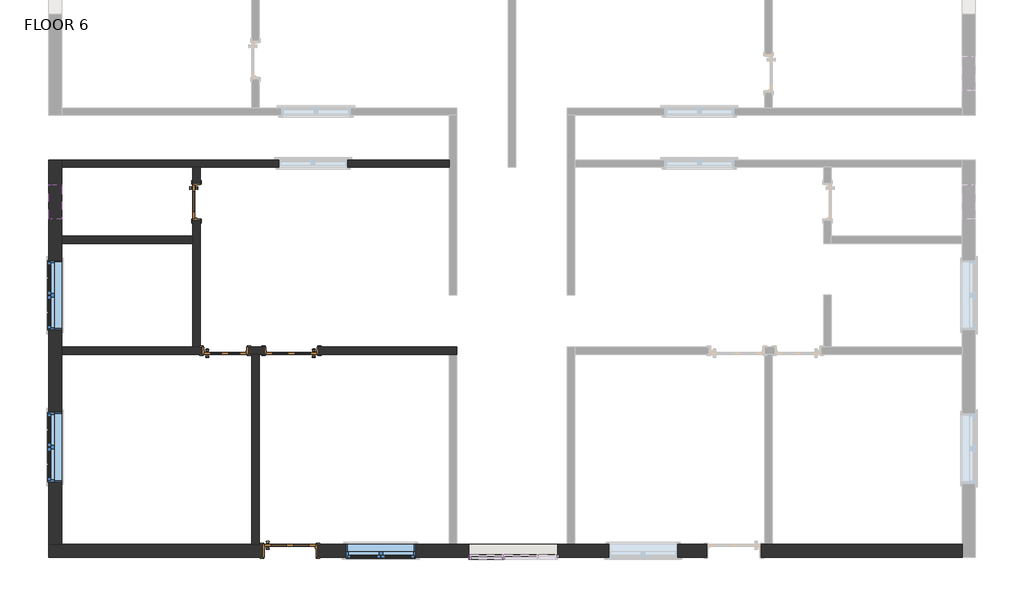
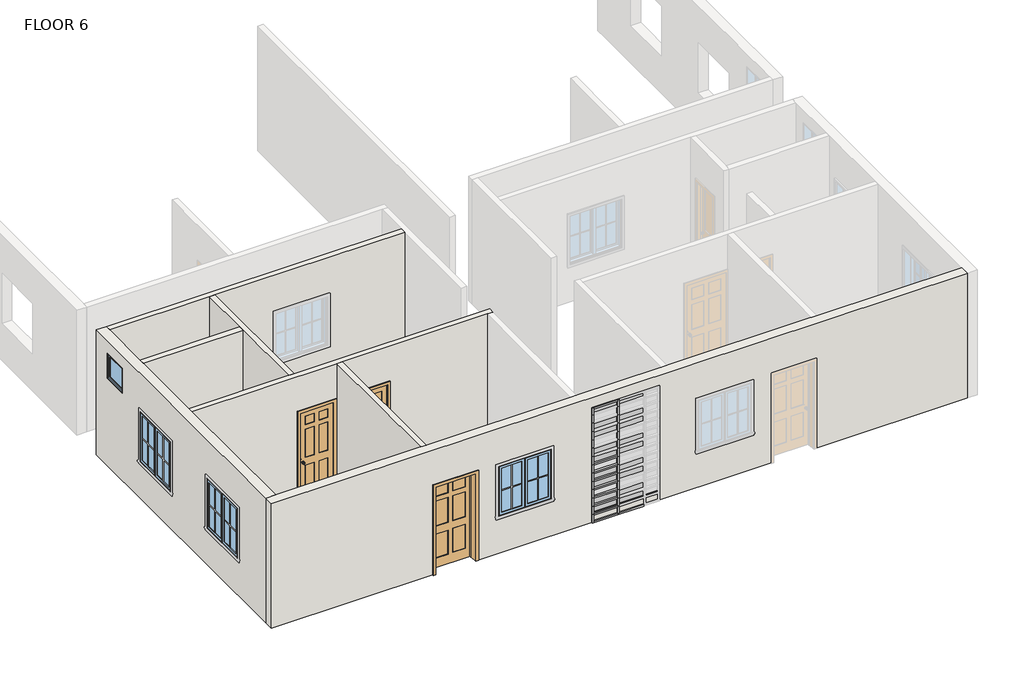
# One storey, part 1 of 4: 38 members, 20 plates, 7 walls, 4 doors, 4 windows.
"""IFC4 building model written with IfcOpenShell, lengths in millimetres."""

from ifc_helpers import new_model, si_unit, frame, origin, place, context, project, spatial, polyline, outline, extrude, faceted_brep, transform, mapped, element, save
from components import door_e337afa5, door_3b50870b, door_d86b6c54, door_03e3dfb5, member_56b223d9, member_a59c64b1, member_fa69921b, member_a67f877f, member_6a7c88b6, member_dc11c383, member_ff422208, system_panel_glazed_844a74e3, system_panel_glazed_a39216e9, system_panel_glazed_b3845325, system_panel_glazed_23b8b45c, system_panel_glazed_26c33eb0, system_panel_glazed_afc0885c, window_80340324, window_9200f5ac

model = new_model("IFC4")

# Units and contexts
model_context = context("Model", 3, world=origin())
ifc_project = project(units=[si_unit("LENGTHUNIT", "METRE", prefix="MILLI")], contexts=[model_context])

# Site, building, storey
site = spatial("IfcSite", under=ifc_project)
building = spatial("IfcBuilding", under=site)
storey = spatial("IfcBuildingStorey", under=building, Name="FLOOR 6", Elevation=9544.3725604)

# Doors
placement = place(None, origin())
door_shape = door_e337afa5(model_context)
element("IfcDoor", 1, ObjectType="Door-Interior-Single-2_Panel-Wood : 24\" x 84\"", at=placement, inside=storey, context=model_context, shape_type="MappedRepresentation", body=[
    mapped(door_shape, transform((-9830.0887331, -1548.6593836, 9544.3725604), x_axis=(0.0, -1.0, 0.0), y_axis=(1.0, 0.0, 0.0), z_axis=(0.0, 0.0, 1.0))),
])
door_2_shape = door_3b50870b(model_context)
element("IfcDoor", 2, ObjectType="Door-Interior-Single-6_Panel-Wood : 30\" x 84\"", at=placement, inside=storey, context=model_context, shape_type="MappedRepresentation", body=[
    mapped(door_2_shape, transform((-9318.9137331, -4180.7343836, 9544.3725604), x_axis=(1.0, 0.0, 0.0), y_axis=(0.0, 1.0, 0.0), z_axis=(0.0, 0.0, 1.0))),
])
door_3_shape = door_d86b6c54(model_context)
element("IfcDoor", 3, ObjectType="Door-Interior-Single-6_Panel-Wood : 36\" x 84\"", at=placement, inside=storey, context=model_context, shape_type="MappedRepresentation", body=[
    mapped(door_3_shape, transform((-8175.9137331, -7704.9843836, 9544.3725604), x_axis=(1.0, 0.0, 0.0), y_axis=(0.0, 1.0, 0.0), z_axis=(0.0, 0.0, 1.0))),
])
door_4_shape = door_03e3dfb5(model_context)
element("IfcDoor", 4, ObjectType="Door-Interior-Single-6_Panel-Wood : 36\" x 84\"", at=placement, inside=storey, context=model_context, shape_type="MappedRepresentation", body=[
    mapped(door_4_shape, transform((-8150.5137331, -4180.7343836, 9544.3725604), x_axis=(-1.0, 0.0, 0.0), y_axis=(0.0, -1.0, 0.0), z_axis=(0.0, 0.0, 1.0))),
])

# Members
member_shape = member_56b223d9(model_context)
element("IfcMember", 5, ObjectType="Rectangular Mullion : 1.5\" x 2.5\" rectangular", at=placement, inside=storey, context=model_context, shape_type="MappedRepresentation", body=[
    mapped(member_shape, transform((-4416.6334597, -7822.4593836, 9544.3725604), x_axis=(1.0, 0.0, 0.0), y_axis=(0.0, -1.0, 0.0), z_axis=(0.0, 0.0, -1.0))),
])
element("IfcMember", 6, ObjectType="Rectangular Mullion : 1.5\" x 2.5\" rectangular", at=placement, inside=storey, context=model_context, shape_type="MappedRepresentation", body=[
    mapped(member_shape, transform((-4416.6334597, -7822.4593836, 9747.5725604), x_axis=(1.0, 0.0, 0.0), y_axis=(0.0, -1.0, 0.0), z_axis=(0.0, 0.0, -1.0))),
])
element("IfcMember", 7, ObjectType="Rectangular Mullion : 1.5\" x 2.5\" rectangular", at=placement, inside=storey, context=model_context, shape_type="MappedRepresentation", body=[
    mapped(member_shape, transform((-4416.6334597, -7822.4593836, 9950.7725604), x_axis=(1.0, 0.0, 0.0), y_axis=(0.0, -1.0, 0.0), z_axis=(0.0, 0.0, -1.0))),
])
element("IfcMember", 8, ObjectType="Rectangular Mullion : 1.5\" x 2.5\" rectangular", at=placement, inside=storey, context=model_context, shape_type="MappedRepresentation", body=[
    mapped(member_shape, transform((-4416.6334597, -7822.4593836, 10153.9725604), x_axis=(1.0, 0.0, 0.0), y_axis=(0.0, -1.0, 0.0), z_axis=(0.0, 0.0, -1.0))),
])
element("IfcMember", 9, ObjectType="Rectangular Mullion : 1.5\" x 2.5\" rectangular", at=placement, inside=storey, context=model_context, shape_type="MappedRepresentation", body=[
    mapped(member_shape, transform((-4416.6334597, -7822.4593836, 10357.1725604), x_axis=(1.0, 0.0, 0.0), y_axis=(0.0, -1.0, 0.0), z_axis=(0.0, 0.0, -1.0))),
])
element("IfcMember", 10, ObjectType="Rectangular Mullion : 1.5\" x 2.5\" rectangular", at=placement, inside=storey, context=model_context, shape_type="MappedRepresentation", body=[
    mapped(member_shape, transform((-4416.6334597, -7822.4593836, 10560.3725604), x_axis=(1.0, 0.0, 0.0), y_axis=(0.0, -1.0, 0.0), z_axis=(0.0, 0.0, -1.0))),
])
element("IfcMember", 11, ObjectType="Rectangular Mullion : 1.5\" x 2.5\" rectangular", at=placement, inside=storey, context=model_context, shape_type="MappedRepresentation", body=[
    mapped(member_shape, transform((-4416.6334597, -7822.4593836, 10763.5725604), x_axis=(1.0, 0.0, 0.0), y_axis=(0.0, -1.0, 0.0), z_axis=(0.0, 0.0, -1.0))),
])
element("IfcMember", 12, ObjectType="Rectangular Mullion : 1.5\" x 2.5\" rectangular", at=placement, inside=storey, context=model_context, shape_type="MappedRepresentation", body=[
    mapped(member_shape, transform((-4416.6334597, -7822.4593836, 10966.7725604), x_axis=(1.0, 0.0, 0.0), y_axis=(0.0, -1.0, 0.0), z_axis=(0.0, 0.0, -1.0))),
])
element("IfcMember", 13, ObjectType="Rectangular Mullion : 1.5\" x 2.5\" rectangular", at=placement, inside=storey, context=model_context, shape_type="MappedRepresentation", body=[
    mapped(member_shape, transform((-4416.6334597, -7822.4593836, 11169.9725604), x_axis=(1.0, 0.0, 0.0), y_axis=(0.0, -1.0, 0.0), z_axis=(0.0, 0.0, -1.0))),
])
element("IfcMember", 14, ObjectType="Rectangular Mullion : 1.5\" x 2.5\" rectangular", at=placement, inside=storey, context=model_context, shape_type="MappedRepresentation", body=[
    mapped(member_shape, transform((-4416.6334597, -7822.4593836, 11373.1725604), x_axis=(1.0, 0.0, 0.0), y_axis=(0.0, -1.0, 0.0), z_axis=(0.0, 0.0, -1.0))),
])
element("IfcMember", 15, ObjectType="Rectangular Mullion : 1.5\" x 2.5\" rectangular", at=placement, inside=storey, context=model_context, shape_type="MappedRepresentation", body=[
    mapped(member_shape, transform((-4416.6334597, -7822.4593836, 11576.3725604), x_axis=(1.0, 0.0, 0.0), y_axis=(0.0, -1.0, 0.0), z_axis=(0.0, 0.0, -1.0))),
])
element("IfcMember", 16, ObjectType="Rectangular Mullion : 1.5\" x 2.5\" rectangular", at=placement, inside=storey, context=model_context, shape_type="MappedRepresentation", body=[
    mapped(member_shape, transform((-4416.6334597, -7822.4593836, 11779.5725604), x_axis=(1.0, 0.0, 0.0), y_axis=(0.0, -1.0, 0.0), z_axis=(0.0, 0.0, -1.0))),
])
element("IfcMember", 17, ObjectType="Rectangular Mullion : 1.5\" x 2.5\" rectangular", at=placement, inside=storey, context=model_context, shape_type="MappedRepresentation", body=[
    mapped(member_shape, transform((-4416.6334597, -7822.4593836, 11982.7725604), x_axis=(1.0, 0.0, 0.0), y_axis=(0.0, -1.0, 0.0), z_axis=(0.0, 0.0, -1.0))),
])
member_2_shape = member_a59c64b1(model_context)
element("IfcMember", 18, ObjectType="Rectangular Mullion : 1.5\" x 2.5\" rectangular", at=placement, inside=storey, context=model_context, shape_type="MappedRepresentation", body=[
    mapped(member_2_shape, transform((-4416.6334597, -7822.4593836, 12185.9725604), x_axis=(1.0, 0.0, 0.0), y_axis=(0.0, -1.0, 0.0), z_axis=(0.0, 0.0, -1.0))),
])
member_3_shape = member_fa69921b(model_context)
element("IfcMember", 19, ObjectType="Rectangular Mullion : 1.5\" x 2.5\" rectangular", at=placement, inside=storey, context=model_context, shape_type="MappedRepresentation", body=[
    mapped(member_3_shape, transform((-4435.6834597, -7822.4593836, 12351.7551755), x_axis=(0.0, 0.0, 1.0), y_axis=(0.0, -1.0, 0.0), z_axis=(1.0, 0.0, 0.0))),
])
element("IfcMember", 20, ObjectType="Rectangular Mullion : 1.5\" x 2.5\" rectangular", at=placement, inside=storey, context=model_context, shape_type="MappedRepresentation", body=[
    mapped(member_3_shape, transform((-4988.13346, -7822.4593836, 9544.3725604), x_axis=(0.0, 0.0, -1.0), y_axis=(0.0, -1.0, 0.0), z_axis=(-1.0, 0.0, 0.0))),
])
member_4_shape = member_a67f877f(model_context)
element("IfcMember", 21, ObjectType="Rectangular Mullion : 1.5\" x 2.5\" rectangular", at=placement, inside=storey, context=model_context, shape_type="MappedRepresentation", body=[
    mapped(member_4_shape, transform((-4397.5834597, -7822.4593836, 9544.3725604), x_axis=(0.0, 0.0, -1.0), y_axis=(0.0, -1.0, 0.0), z_axis=(-1.0, 0.0, 0.0))),
])
member_5_shape = member_6a7c88b6(model_context)
element("IfcMember", 22, ObjectType="Rectangular Mullion : 1.5\" x 2.5\" rectangular", at=placement, inside=storey, context=model_context, shape_type="MappedRepresentation", body=[
    mapped(member_5_shape, transform((-4435.6834597, -7822.4593836, 9747.5725604), x_axis=(0.0, 0.0, 1.0), y_axis=(0.0, -1.0, 0.0), z_axis=(1.0, 0.0, 0.0))),
])
element("IfcMember", 23, ObjectType="Rectangular Mullion : 1.5\" x 2.5\" rectangular", at=placement, inside=storey, context=model_context, shape_type="MappedRepresentation", body=[
    mapped(member_5_shape, transform((-4435.6834597, -7822.4593836, 9950.7725604), x_axis=(0.0, 0.0, 1.0), y_axis=(0.0, -1.0, 0.0), z_axis=(1.0, 0.0, 0.0))),
])
element("IfcMember", 24, ObjectType="Rectangular Mullion : 1.5\" x 2.5\" rectangular", at=placement, inside=storey, context=model_context, shape_type="MappedRepresentation", body=[
    mapped(member_5_shape, transform((-4435.6834597, -7822.4593836, 10153.9725604), x_axis=(0.0, 0.0, 1.0), y_axis=(0.0, -1.0, 0.0), z_axis=(1.0, 0.0, 0.0))),
])
element("IfcMember", 25, ObjectType="Rectangular Mullion : 1.5\" x 2.5\" rectangular", at=placement, inside=storey, context=model_context, shape_type="MappedRepresentation", body=[
    mapped(member_5_shape, transform((-4435.6834597, -7822.4593836, 10357.1725604), x_axis=(0.0, 0.0, 1.0), y_axis=(0.0, -1.0, 0.0), z_axis=(1.0, 0.0, 0.0))),
])
element("IfcMember", 26, ObjectType="Rectangular Mullion : 1.5\" x 2.5\" rectangular", at=placement, inside=storey, context=model_context, shape_type="MappedRepresentation", body=[
    mapped(member_5_shape, transform((-4435.6834597, -7822.4593836, 10560.3725604), x_axis=(0.0, 0.0, 1.0), y_axis=(0.0, -1.0, 0.0), z_axis=(1.0, 0.0, 0.0))),
])
element("IfcMember", 27, ObjectType="Rectangular Mullion : 1.5\" x 2.5\" rectangular", at=placement, inside=storey, context=model_context, shape_type="MappedRepresentation", body=[
    mapped(member_5_shape, transform((-4435.6834597, -7822.4593836, 10763.5725604), x_axis=(0.0, 0.0, 1.0), y_axis=(0.0, -1.0, 0.0), z_axis=(1.0, 0.0, 0.0))),
])
element("IfcMember", 28, ObjectType="Rectangular Mullion : 1.5\" x 2.5\" rectangular", at=placement, inside=storey, context=model_context, shape_type="MappedRepresentation", body=[
    mapped(member_5_shape, transform((-4435.6834597, -7822.4593836, 10966.7725604), x_axis=(0.0, 0.0, 1.0), y_axis=(0.0, -1.0, 0.0), z_axis=(1.0, 0.0, 0.0))),
])
member_6_shape = member_dc11c383(model_context)
element("IfcMember", 29, ObjectType="Rectangular Mullion : 1.5\" x 2.5\" rectangular", at=placement, inside=storey, context=model_context, shape_type="MappedRepresentation", body=[
    mapped(member_6_shape, transform((-5026.23346, -7822.4593836, 12351.7551755), x_axis=(-1.0, 0.0, 0.0), y_axis=(0.0, -1.0, 0.0), z_axis=(0.0, 0.0, 1.0))),
])
member_7_shape = member_ff422208(model_context)
element("IfcMember", 30, ObjectType="Rectangular Mullion : 1.5\" x 2.5\" rectangular", at=placement, inside=storey, context=model_context, shape_type="MappedRepresentation", body=[
    mapped(member_7_shape, transform((-5026.23346, -7822.4593836, 9747.5725604), x_axis=(-1.0, 0.0, 0.0), y_axis=(0.0, -1.0, 0.0), z_axis=(0.0, 0.0, 1.0))),
])
element("IfcMember", 31, ObjectType="Rectangular Mullion : 1.5\" x 2.5\" rectangular", at=placement, inside=storey, context=model_context, shape_type="MappedRepresentation", body=[
    mapped(member_7_shape, transform((-5026.23346, -7822.4593836, 9950.7725604), x_axis=(-1.0, 0.0, 0.0), y_axis=(0.0, -1.0, 0.0), z_axis=(0.0, 0.0, 1.0))),
])
element("IfcMember", 32, ObjectType="Rectangular Mullion : 1.5\" x 2.5\" rectangular", at=placement, inside=storey, context=model_context, shape_type="MappedRepresentation", body=[
    mapped(member_7_shape, transform((-5026.23346, -7822.4593836, 10153.9725604), x_axis=(-1.0, 0.0, 0.0), y_axis=(0.0, -1.0, 0.0), z_axis=(0.0, 0.0, 1.0))),
])
element("IfcMember", 33, ObjectType="Rectangular Mullion : 1.5\" x 2.5\" rectangular", at=placement, inside=storey, context=model_context, shape_type="MappedRepresentation", body=[
    mapped(member_7_shape, transform((-5026.23346, -7822.4593836, 10357.1725604), x_axis=(-1.0, 0.0, 0.0), y_axis=(0.0, -1.0, 0.0), z_axis=(0.0, 0.0, 1.0))),
])
element("IfcMember", 34, ObjectType="Rectangular Mullion : 1.5\" x 2.5\" rectangular", at=placement, inside=storey, context=model_context, shape_type="MappedRepresentation", body=[
    mapped(member_7_shape, transform((-5026.23346, -7822.4593836, 10560.3725604), x_axis=(-1.0, 0.0, 0.0), y_axis=(0.0, -1.0, 0.0), z_axis=(0.0, 0.0, 1.0))),
])
element("IfcMember", 35, ObjectType="Rectangular Mullion : 1.5\" x 2.5\" rectangular", at=placement, inside=storey, context=model_context, shape_type="MappedRepresentation", body=[
    mapped(member_7_shape, transform((-5026.23346, -7822.4593836, 10763.5725604), x_axis=(-1.0, 0.0, 0.0), y_axis=(0.0, -1.0, 0.0), z_axis=(0.0, 0.0, 1.0))),
])
element("IfcMember", 36, ObjectType="Rectangular Mullion : 1.5\" x 2.5\" rectangular", at=placement, inside=storey, context=model_context, shape_type="MappedRepresentation", body=[
    mapped(member_7_shape, transform((-5026.23346, -7822.4593836, 10966.7725604), x_axis=(-1.0, 0.0, 0.0), y_axis=(0.0, -1.0, 0.0), z_axis=(0.0, 0.0, 1.0))),
])
element("IfcMember", 37, ObjectType="Rectangular Mullion : 1.5\" x 2.5\" rectangular", at=placement, inside=storey, context=model_context, shape_type="MappedRepresentation", body=[
    mapped(member_7_shape, transform((-5026.23346, -7822.4593836, 11169.9725604), x_axis=(-1.0, 0.0, 0.0), y_axis=(0.0, -1.0, 0.0), z_axis=(0.0, 0.0, 1.0))),
])
element("IfcMember", 38, ObjectType="Rectangular Mullion : 1.5\" x 2.5\" rectangular", at=placement, inside=storey, context=model_context, shape_type="MappedRepresentation", body=[
    mapped(member_7_shape, transform((-5026.23346, -7822.4593836, 11373.1725604), x_axis=(-1.0, 0.0, 0.0), y_axis=(0.0, -1.0, 0.0), z_axis=(0.0, 0.0, 1.0))),
])
element("IfcMember", 39, ObjectType="Rectangular Mullion : 1.5\" x 2.5\" rectangular", at=placement, inside=storey, context=model_context, shape_type="MappedRepresentation", body=[
    mapped(member_7_shape, transform((-5026.23346, -7822.4593836, 11576.3725604), x_axis=(-1.0, 0.0, 0.0), y_axis=(0.0, -1.0, 0.0), z_axis=(0.0, 0.0, 1.0))),
])
element("IfcMember", 40, ObjectType="Rectangular Mullion : 1.5\" x 2.5\" rectangular", at=placement, inside=storey, context=model_context, shape_type="MappedRepresentation", body=[
    mapped(member_7_shape, transform((-5026.23346, -7822.4593836, 11779.5725604), x_axis=(-1.0, 0.0, 0.0), y_axis=(0.0, -1.0, 0.0), z_axis=(0.0, 0.0, 1.0))),
])
element("IfcMember", 41, ObjectType="Rectangular Mullion : 1.5\" x 2.5\" rectangular", at=placement, inside=storey, context=model_context, shape_type="MappedRepresentation", body=[
    mapped(member_7_shape, transform((-5026.23346, -7822.4593836, 11982.7725604), x_axis=(-1.0, 0.0, 0.0), y_axis=(0.0, -1.0, 0.0), z_axis=(0.0, 0.0, 1.0))),
])
element("IfcMember", 42, ObjectType="Rectangular Mullion : 1.5\" x 2.5\" rectangular", at=placement, inside=storey, context=model_context, shape_type="MappedRepresentation", body=[
    mapped(member_7_shape, transform((-5026.23346, -7822.4593836, 12185.9725604), x_axis=(-1.0, 0.0, 0.0), y_axis=(0.0, -1.0, 0.0), z_axis=(0.0, 0.0, 1.0))),
])

# Plates
system_panel_glazed_shape = system_panel_glazed_844a74e3(model_context)
element("IfcPlate", 43, ObjectType="System Panel : Glazed", at=placement, inside=storey, context=model_context, shape_type="MappedRepresentation", body=[
    mapped(system_panel_glazed_shape, transform((-4711.9084599, -7822.4593836, 9582.4725604), x_axis=(1.0, 0.0, 0.0), y_axis=(0.0, 1.0, 0.0), z_axis=(0.0, 0.0, 1.0))),
])
system_panel_glazed_2_shape = system_panel_glazed_a39216e9(model_context)
element("IfcPlate", 44, ObjectType="System Panel : Glazed", at=placement, inside=storey, context=model_context, shape_type="MappedRepresentation", body=[
    mapped(system_panel_glazed_2_shape, transform((-4111.8334597, -7822.4593836, 9582.4725604), x_axis=(1.0, 0.0, 0.0), y_axis=(0.0, 1.0, 0.0), z_axis=(0.0, 0.0, 1.0))),
])
system_panel_glazed_3_shape = system_panel_glazed_b3845325(model_context)
element("IfcPlate", 45, ObjectType="System Panel : Glazed", at=placement, inside=storey, context=model_context, shape_type="MappedRepresentation", body=[
    mapped(system_panel_glazed_3_shape, transform((-4711.9084599, -7822.4593836, 9766.6225604), x_axis=(1.0, 0.0, 0.0), y_axis=(0.0, 1.0, 0.0), z_axis=(0.0, 0.0, 1.0))),
])
element("IfcPlate", 46, ObjectType="System Panel : Glazed", at=placement, inside=storey, context=model_context, shape_type="MappedRepresentation", body=[
    mapped(system_panel_glazed_3_shape, transform((-4711.9084599, -7822.4593836, 9969.8225604), x_axis=(1.0, 0.0, 0.0), y_axis=(0.0, 1.0, 0.0), z_axis=(0.0, 0.0, 1.0))),
])
element("IfcPlate", 47, ObjectType="System Panel : Glazed", at=placement, inside=storey, context=model_context, shape_type="MappedRepresentation", body=[
    mapped(system_panel_glazed_3_shape, transform((-4711.9084599, -7822.4593836, 10376.2225604), x_axis=(1.0, 0.0, 0.0), y_axis=(0.0, 1.0, 0.0), z_axis=(0.0, 0.0, 1.0))),
])
element("IfcPlate", 48, ObjectType="System Panel : Glazed", at=placement, inside=storey, context=model_context, shape_type="MappedRepresentation", body=[
    mapped(system_panel_glazed_3_shape, transform((-4711.9084599, -7822.4593836, 10579.4225604), x_axis=(1.0, 0.0, 0.0), y_axis=(0.0, 1.0, 0.0), z_axis=(0.0, 0.0, 1.0))),
])
element("IfcPlate", 49, ObjectType="System Panel : Glazed", at=placement, inside=storey, context=model_context, shape_type="MappedRepresentation", body=[
    mapped(system_panel_glazed_3_shape, transform((-4711.9084599, -7822.4593836, 10985.8225604), x_axis=(1.0, 0.0, 0.0), y_axis=(0.0, 1.0, 0.0), z_axis=(0.0, 0.0, 1.0))),
])
element("IfcPlate", 50, ObjectType="System Panel : Glazed", at=placement, inside=storey, context=model_context, shape_type="MappedRepresentation", body=[
    mapped(system_panel_glazed_3_shape, transform((-4711.9084599, -7822.4593836, 11189.0225604), x_axis=(1.0, 0.0, 0.0), y_axis=(0.0, 1.0, 0.0), z_axis=(0.0, 0.0, 1.0))),
])
element("IfcPlate", 51, ObjectType="System Panel : Glazed", at=placement, inside=storey, context=model_context, shape_type="MappedRepresentation", body=[
    mapped(system_panel_glazed_3_shape, transform((-4711.9084599, -7822.4593836, 11595.4225604), x_axis=(1.0, 0.0, 0.0), y_axis=(0.0, 1.0, 0.0), z_axis=(0.0, 0.0, 1.0))),
])
element("IfcPlate", 52, ObjectType="System Panel : Glazed", at=placement, inside=storey, context=model_context, shape_type="MappedRepresentation", body=[
    mapped(system_panel_glazed_3_shape, transform((-4711.9084599, -7822.4593836, 11798.6225604), x_axis=(1.0, 0.0, 0.0), y_axis=(0.0, 1.0, 0.0), z_axis=(0.0, 0.0, 1.0))),
])
system_panel_glazed_4_shape = system_panel_glazed_23b8b45c(model_context)
element("IfcPlate", 53, ObjectType="System Panel : Glazed", at=placement, inside=storey, context=model_context, shape_type="MappedRepresentation", body=[
    mapped(system_panel_glazed_4_shape, transform((-4111.8334597, -7822.4593836, 9766.6225604), x_axis=(1.0, 0.0, 0.0), y_axis=(0.0, 1.0, 0.0), z_axis=(0.0, 0.0, 1.0))),
])
element("IfcPlate", 54, ObjectType="System Panel : Glazed", at=placement, inside=storey, context=model_context, shape_type="MappedRepresentation", body=[
    mapped(system_panel_glazed_4_shape, transform((-4111.8334597, -7822.4593836, 9969.8225604), x_axis=(1.0, 0.0, 0.0), y_axis=(0.0, 1.0, 0.0), z_axis=(0.0, 0.0, 1.0))),
])
element("IfcPlate", 55, ObjectType="System Panel : Glazed", at=placement, inside=storey, context=model_context, shape_type="MappedRepresentation", body=[
    mapped(system_panel_glazed_4_shape, transform((-4111.8334597, -7822.4593836, 10376.2225604), x_axis=(1.0, 0.0, 0.0), y_axis=(0.0, 1.0, 0.0), z_axis=(0.0, 0.0, 1.0))),
])
element("IfcPlate", 56, ObjectType="System Panel : Glazed", at=placement, inside=storey, context=model_context, shape_type="MappedRepresentation", body=[
    mapped(system_panel_glazed_4_shape, transform((-4111.8334597, -7822.4593836, 10579.4225604), x_axis=(1.0, 0.0, 0.0), y_axis=(0.0, 1.0, 0.0), z_axis=(0.0, 0.0, 1.0))),
])
element("IfcPlate", 57, ObjectType="System Panel : Glazed", at=placement, inside=storey, context=model_context, shape_type="MappedRepresentation", body=[
    mapped(system_panel_glazed_4_shape, transform((-4111.8334597, -7822.4593836, 10985.8225604), x_axis=(1.0, 0.0, 0.0), y_axis=(0.0, 1.0, 0.0), z_axis=(0.0, 0.0, 1.0))),
])
element("IfcPlate", 58, ObjectType="System Panel : Glazed", at=placement, inside=storey, context=model_context, shape_type="MappedRepresentation", body=[
    mapped(system_panel_glazed_4_shape, transform((-4111.8334597, -7822.4593836, 11189.0225604), x_axis=(1.0, 0.0, 0.0), y_axis=(0.0, 1.0, 0.0), z_axis=(0.0, 0.0, 1.0))),
])
element("IfcPlate", 59, ObjectType="System Panel : Glazed", at=placement, inside=storey, context=model_context, shape_type="MappedRepresentation", body=[
    mapped(system_panel_glazed_4_shape, transform((-4111.8334597, -7822.4593836, 11595.4225604), x_axis=(1.0, 0.0, 0.0), y_axis=(0.0, 1.0, 0.0), z_axis=(0.0, 0.0, 1.0))),
])
element("IfcPlate", 60, ObjectType="System Panel : Glazed", at=placement, inside=storey, context=model_context, shape_type="MappedRepresentation", body=[
    mapped(system_panel_glazed_4_shape, transform((-4111.8334597, -7822.4593836, 11798.6225604), x_axis=(1.0, 0.0, 0.0), y_axis=(0.0, 1.0, 0.0), z_axis=(0.0, 0.0, 1.0))),
])
system_panel_glazed_5_shape = system_panel_glazed_26c33eb0(model_context)
element("IfcPlate", 61, ObjectType="System Panel : Glazed", at=placement, inside=storey, context=model_context, shape_type="MappedRepresentation", body=[
    mapped(system_panel_glazed_5_shape, transform((-4711.9084599, -7822.4593836, 12205.0225604), x_axis=(1.0, 0.0, 0.0), y_axis=(0.0, 1.0, 0.0), z_axis=(0.0, 0.0, 1.0))),
])
system_panel_glazed_6_shape = system_panel_glazed_afc0885c(model_context)
element("IfcPlate", 62, ObjectType="System Panel : Glazed", at=placement, inside=storey, context=model_context, shape_type="MappedRepresentation", body=[
    mapped(system_panel_glazed_6_shape, transform((-4111.8334597, -7822.4593836, 12205.0225604), x_axis=(1.0, 0.0, 0.0), y_axis=(0.0, 1.0, 0.0), z_axis=(0.0, 0.0, 1.0))),
])

# Walls
element("IfcWall", 63, ObjectType="Inner Wall 5\"", at=placement, inside=storey, context=model_context, shape_type="Brep", body=[
    faceted_brep([(-12201.8137331, -939.0593836, 9544.3725604), (-9890.4137331, -939.0593836, 9544.3725604), (-9763.4137331, -939.0593836, 9544.3725604), (-5369.2137331, -939.0593836, 9544.3725604), (-5369.2137331, -939.0593836, 12592.3725604), (-9763.4137331, -939.0593836, 12592.3725604), (-9890.4137331, -939.0593836, 12592.3725604), (-12201.8137331, -939.0593836, 12592.3725604), (-7159.9137331, -939.0593836, 11677.9725604), (-7159.9137331, -939.0593836, 10458.7725604), (-8379.1137331, -939.0593836, 10458.7725604), (-8379.1137331, -939.0593836, 11677.9725604), (-12201.8137331, -812.0593836, 9544.3725604), (-12201.8137331, -812.0593836, 12592.3725604), (-5369.2137331, -812.0593836, 12592.3725604), (-5369.2137331, -812.0593836, 9544.3725604), (-7159.9137331, -812.0593836, 11677.9725604), (-8379.1137331, -812.0593836, 11677.9725604), (-8379.1137331, -812.0593836, 10458.7725604), (-7159.9137331, -812.0593836, 10458.7725604)], [[[0, 1, 2, 3, 4, 5, 6, 7], [8, 9, 10, 11]], [[12, 13, 14, 15], [16, 17, 18, 19]], [[3, 2, 1, 0, 12, 15]], [[7, 6, 5, 4, 14, 13]], [[0, 7, 13, 12]], [[4, 3, 15, 14]], [[9, 8, 16, 19]], [[10, 9, 19, 18]], [[11, 10, 18, 17]], [[8, 11, 17, 16]]]),
])
element("IfcWall", 64, ObjectType="Inner Wall 5\"", at=placement, inside=storey, context=model_context, shape_type="SweptSolid", body=[
    extrude(outline(polyline([(-8722.0137331, -4241.0593836), (-8722.0137331, -7593.8593836), (-8849.0137331, -7593.8593836), (-8849.0137331, -4241.0593836), (-8722.0137331, -4241.0593836)])), frame((0.0, 0.0, 9544.3725604), z_axis=(0.0, 0.0, 1.0), x_axis=(1.0, 0.0, 0.0)), (0.0, 0.0, 1.0), 3048.0),
])
element("IfcWall", 65, ObjectType="Inner Wall 5\"", at=placement, inside=storey, context=model_context, shape_type="Brep", body=[
    faceted_brep([(-12201.8137331, -4114.0593836, 12592.3725604), (-9890.4137331, -4114.0593836, 12592.3725604), (-9763.4137331, -4114.0593836, 12592.3725604), (-5242.2137331, -4114.0593836, 12592.3725604), (-5242.2137331, -4114.0593836, 9544.3725604), (-7667.9137331, -4114.0593836, 9544.3725604), (-7667.9137331, -4114.0593836, 11703.3725604), (-8633.1137331, -4114.0593836, 11703.3725604), (-8633.1137331, -4114.0593836, 9544.3725604), (-8912.5137331, -4114.0593836, 9544.3725604), (-8912.5137331, -4114.0593836, 11703.3725604), (-9725.3137331, -4114.0593836, 11703.3725604), (-9725.3137331, -4114.0593836, 9544.3725604), (-9763.4137331, -4114.0593836, 9544.3725604), (-9890.4137331, -4114.0593836, 9544.3725604), (-12201.8137331, -4114.0593836, 9544.3725604), (-5242.2137331, -4241.0593836, 12592.3725604), (-5369.2137331, -4241.0593836, 12592.3725604), (-8722.0137331, -4241.0593836, 12592.3725604), (-8849.0137331, -4241.0593836, 12592.3725604), (-12201.8137331, -4241.0593836, 12592.3725604), (-12201.8137331, -4241.0593836, 9544.3725604), (-9725.3137331, -4241.0593836, 9544.3725604), (-9725.3137331, -4241.0593836, 11703.3725604), (-8912.5137331, -4241.0593836, 11703.3725604), (-8912.5137331, -4241.0593836, 9544.3725604), (-8849.0137331, -4241.0593836, 9544.3725604), (-8722.0137331, -4241.0593836, 9544.3725604), (-8633.1137331, -4241.0593836, 9544.3725604), (-8633.1137331, -4241.0593836, 11703.3725604), (-7667.9137331, -4241.0593836, 11703.3725604), (-7667.9137331, -4241.0593836, 9544.3725604), (-5369.2137331, -4241.0593836, 9544.3725604), (-5242.2137331, -4241.0593836, 9544.3725604)], [[[0, 1, 2, 3, 4, 5, 6, 7, 8, 9, 10, 11, 12, 13, 14, 15]], [[16, 17, 18, 19, 20, 21, 22, 23, 24, 25, 26, 27, 28, 29, 30, 31, 32, 33]], [[21, 15, 14, 13, 12, 22]], [[4, 33, 32, 31, 5]], [[25, 9, 8, 28, 27, 26]], [[3, 2, 1, 0, 20, 19, 18, 17, 16]], [[0, 15, 21, 20]], [[4, 3, 16, 33]], [[10, 9, 25, 24]], [[11, 10, 24, 23]], [[12, 11, 23, 22]], [[7, 29, 28, 8]], [[29, 7, 6, 30]], [[30, 6, 5, 31]]]),
])
element("IfcWall", 66, ObjectType="Inner Wall 5\"", at=placement, inside=storey, context=model_context, shape_type="Brep", body=[
    faceted_brep([(-9763.4137331, -939.0593836, 12592.3725604), (-9763.4137331, -4114.0593836, 12592.3725604), (-9763.4137331, -4114.0593836, 9544.3725604), (-9763.4137331, -1878.8593836, 9544.3725604), (-9763.4137331, -1878.8593836, 11703.3725604), (-9763.4137331, -1218.4593836, 11703.3725604), (-9763.4137331, -1218.4593836, 9544.3725604), (-9763.4137331, -939.0593836, 9544.3725604), (-9890.4137331, -4114.0593836, 12592.3725604), (-9890.4137331, -2285.2593836, 12592.3725604), (-9890.4137331, -2158.2593836, 12592.3725604), (-9890.4137331, -939.0593836, 12592.3725604), (-9890.4137331, -939.0593836, 9544.3725604), (-9890.4137331, -1218.4593836, 9544.3725604), (-9890.4137331, -1218.4593836, 11703.3725604), (-9890.4137331, -1878.8593836, 11703.3725604), (-9890.4137331, -1878.8593836, 9544.3725604), (-9890.4137331, -2158.2593836, 9544.3725604), (-9890.4137331, -2285.2593836, 9544.3725604), (-9890.4137331, -4114.0593836, 9544.3725604)], [[[0, 1, 2, 3, 4, 5, 6, 7]], [[8, 9, 10, 11, 12, 13, 14, 15, 16, 17, 18, 19]], [[2, 19, 18, 17, 16, 3]], [[12, 7, 6, 13]], [[1, 0, 11, 10, 9, 8]], [[2, 1, 8, 19]], [[0, 7, 12, 11]], [[15, 4, 3, 16]], [[4, 15, 14, 5]], [[5, 14, 13, 6]]]),
])
element("IfcWall", 67, ObjectType="Inner Wall 5\"", at=placement, inside=storey, context=model_context, shape_type="SweptSolid", body=[
    extrude(outline(polyline([(-12201.8137331, -2158.2593836), (-9890.4137331, -2158.2593836), (-9890.4137331, -2285.2593836), (-12201.8137331, -2285.2593836), (-12201.8137331, -2158.2593836)])), frame((0.0, 0.0, 9544.3725604), z_axis=(0.0, 0.0, 1.0), x_axis=(1.0, 0.0, 0.0)), (0.0, 0.0, 1.0), 3048.0),
])
element("IfcWall", 68, ObjectType="outer wall 9\"", at=placement, inside=storey, context=model_context, shape_type="Brep", body=[
    faceted_brep([(3673.1862669, -7822.4593836, 12592.3725604), (-12430.4137331, -7822.4593836, 12592.3725604), (-12430.4137331, -7822.4593836, 9544.3725604), (-8658.5137331, -7822.4593836, 9544.3725604), (-8658.5137331, -7822.4593836, 11703.3725604), (-7693.3137331, -7822.4593836, 11703.3725604), (-7693.3137331, -7822.4593836, 9544.3725604), (-835.3137331, -7822.4593836, 9544.3725604), (-835.3137331, -7822.4593836, 11703.3725604), (129.8862669, -7822.4593836, 11703.3725604), (129.8862669, -7822.4593836, 9544.3725604), (3673.1862669, -7822.4593836, 9544.3725604), (-2562.5137331, -7822.4593836, 11677.9725604), (-1343.3137331, -7822.4593836, 11677.9725604), (-1343.3137331, -7822.4593836, 10458.7725604), (-2562.5137331, -7822.4593836, 10458.7725604), (-7185.3137331, -7822.4593836, 11677.9725604), (-5966.1137331, -7822.4593836, 11677.9725604), (-5966.1137331, -7822.4593836, 10458.7725604), (-7185.3137331, -7822.4593836, 10458.7725604), (-5026.23346, -7822.4593836, 12351.7551755), (-3461.6513929, -7822.4593836, 12351.7551755), (-3461.6513929, -7822.4593836, 9778.8868874), (-5026.23346, -7822.4593836, 9778.8868874), (-12430.4137331, -7593.8593836, 12592.3725604), (-12201.8137331, -7593.8593836, 12592.3725604), (-8849.0137331, -7593.8593836, 12592.3725604), (-8722.0137331, -7593.8593836, 12592.3725604), (-5369.2137331, -7593.8593836, 12592.3725604), (-5242.2137331, -7593.8593836, 12592.3725604), (-3286.4137331, -7593.8593836, 12592.3725604), (-3159.4137331, -7593.8593836, 12592.3725604), (193.3862669, -7593.8593836, 12592.3725604), (320.3862669, -7593.8593836, 12592.3725604), (3673.1862669, -7593.8593836, 12592.3725604), (3673.1862669, -7593.8593836, 9544.3725604), (320.3862669, -7593.8593836, 9544.3725604), (193.3862669, -7593.8593836, 9544.3725604), (129.8862669, -7593.8593836, 9544.3725604), (129.8862669, -7593.8593836, 11703.3725604), (-835.3137331, -7593.8593836, 11703.3725604), (-835.3137331, -7593.8593836, 9544.3725604), (-3159.4137331, -7593.8593836, 9544.3725604), (-3286.4137331, -7593.8593836, 9544.3725604), (-5242.2137331, -7593.8593836, 9544.3725604), (-5369.2137331, -7593.8593836, 9544.3725604), (-7693.3137331, -7593.8593836, 9544.3725604), (-7693.3137331, -7593.8593836, 11703.3725604), (-8658.5137331, -7593.8593836, 11703.3725604), (-8658.5137331, -7593.8593836, 9544.3725604), (-8722.0137331, -7593.8593836, 9544.3725604), (-8849.0137331, -7593.8593836, 9544.3725604), (-12201.8137331, -7593.8593836, 9544.3725604), (-12430.4137331, -7593.8593836, 9544.3725604), (-2562.5137331, -7593.8593836, 11677.9725604), (-2562.5137331, -7593.8593836, 10458.7725604), (-1343.3137331, -7593.8593836, 10458.7725604), (-1343.3137331, -7593.8593836, 11677.9725604), (-7185.3137331, -7593.8593836, 11677.9725604), (-7185.3137331, -7593.8593836, 10458.7725604), (-5966.1137331, -7593.8593836, 10458.7725604), (-5966.1137331, -7593.8593836, 11677.9725604), (-3461.6513929, -7593.8593836, 12351.7551755), (-5026.23346, -7593.8593836, 12351.7551755), (-5026.23346, -7593.8593836, 9778.8868874), (-3461.6513929, -7593.8593836, 9778.8868874)], [[[0, 1, 2, 3, 4, 5, 6, 7, 8, 9, 10, 11], [12, 13, 14, 15], [16, 17, 18, 19], [20, 21, 22, 23]], [[24, 25, 26, 27, 28, 29, 30, 31, 32, 33, 34, 35, 36, 37, 38, 39, 40, 41, 42, 43, 44, 45, 46, 47, 48, 49, 50, 51, 52, 53], [54, 55, 56, 57], [58, 59, 60, 61], [62, 63, 64, 65]], [[2, 53, 52, 51, 50, 49, 3]], [[35, 11, 10, 38, 37, 36]], [[6, 46, 45, 44, 43, 42, 41, 7]], [[1, 0, 34, 33, 32, 31, 30, 29, 28, 27, 26, 25, 24]], [[2, 1, 24, 53]], [[0, 11, 35, 34]], [[5, 47, 46, 6]], [[47, 5, 4, 48]], [[48, 4, 3, 49]], [[40, 8, 7, 41]], [[8, 40, 39, 9]], [[9, 39, 38, 10]], [[55, 54, 12, 15]], [[56, 55, 15, 14]], [[57, 56, 14, 13]], [[54, 57, 13, 12]], [[59, 58, 16, 19]], [[60, 59, 19, 18]], [[61, 60, 18, 17]], [[58, 61, 17, 16]], [[20, 63, 62, 21]], [[22, 65, 64, 23]], [[63, 20, 23, 64]], [[21, 62, 65, 22]]]),
])
element("IfcWall", 69, ObjectType="outer wall 9\"", at=placement, inside=storey, context=model_context, shape_type="Brep", body=[
    faceted_brep([(-12430.4137331, -812.0593836, 9544.3725604), (-12430.4137331, -7593.8593836, 9544.3725604), (-12430.4137331, -7593.8593836, 12592.3725604), (-12430.4137331, -812.0593836, 12592.3725604), (-12430.4137331, -5269.7593836, 11677.9725604), (-12430.4137331, -6488.9593836, 11677.9725604), (-12430.4137331, -6488.9593836, 10458.7725604), (-12430.4137331, -5269.7593836, 10458.7725604), (-12430.4137331, -2590.0593836, 11677.9725604), (-12430.4137331, -3809.2593836, 11677.9725604), (-12430.4137331, -3809.2593836, 10458.7725604), (-12430.4137331, -2590.0593836, 10458.7725604), (-12430.4137331, -1243.8593836, 12287.5725604), (-12430.4137331, -1853.4593836, 12287.5725604), (-12430.4137331, -1853.4593836, 11677.9725604), (-12430.4137331, -1243.8593836, 11677.9725604), (-12201.8137331, -812.0593836, 9544.3725604), (-12201.8137331, -812.0593836, 12592.3725604), (-12201.8137331, -939.0593836, 12592.3725604), (-12201.8137331, -2158.2593836, 12592.3725604), (-12201.8137331, -2285.2593836, 12592.3725604), (-12201.8137331, -4114.0593836, 12592.3725604), (-12201.8137331, -4241.0593836, 12592.3725604), (-12201.8137331, -7593.8593836, 12592.3725604), (-12201.8137331, -7593.8593836, 9544.3725604), (-12201.8137331, -4241.0593836, 9544.3725604), (-12201.8137331, -4114.0593836, 9544.3725604), (-12201.8137331, -2285.2593836, 9544.3725604), (-12201.8137331, -2158.2593836, 9544.3725604), (-12201.8137331, -939.0593836, 9544.3725604), (-12201.8137331, -5269.7593836, 11677.9725604), (-12201.8137331, -5269.7593836, 10458.7725604), (-12201.8137331, -6488.9593836, 10458.7725604), (-12201.8137331, -6488.9593836, 11677.9725604), (-12201.8137331, -2590.0593836, 11677.9725604), (-12201.8137331, -2590.0593836, 10458.7725604), (-12201.8137331, -3809.2593836, 10458.7725604), (-12201.8137331, -3809.2593836, 11677.9725604), (-12201.8137331, -1243.8593836, 12287.5725604), (-12201.8137331, -1243.8593836, 11677.9725604), (-12201.8137331, -1853.4593836, 11677.9725604), (-12201.8137331, -1853.4593836, 12287.5725604)], [[[0, 1, 2, 3], [4, 5, 6, 7], [8, 9, 10, 11], [12, 13, 14, 15]], [[16, 17, 18, 19, 20, 21, 22, 23, 24, 25, 26, 27, 28, 29], [30, 31, 32, 33], [34, 35, 36, 37], [38, 39, 40, 41]], [[1, 0, 16, 29, 28, 27, 26, 25, 24]], [[3, 2, 23, 22, 21, 20, 19, 18, 17]], [[2, 1, 24, 23]], [[0, 3, 17, 16]], [[31, 30, 4, 7]], [[32, 31, 7, 6]], [[33, 32, 6, 5]], [[30, 33, 5, 4]], [[35, 34, 8, 11]], [[36, 35, 11, 10]], [[37, 36, 10, 9]], [[34, 37, 9, 8]], [[39, 38, 12, 15]], [[40, 39, 15, 14]], [[41, 40, 14, 13]], [[38, 41, 13, 12]]]),
])

# Windows
window_shape = window_80340324(model_context)
element("IfcWindow", 70, ObjectType="Fixed : 24\" x 24\"", at=placement, inside=storey, context=model_context, shape_type="MappedRepresentation", body=[
    mapped(window_shape, transform((-12316.1137331, -1510.5593836, 10763.5725604), x_axis=(0.0, 1.0, 0.0), y_axis=(-1.0, 0.0, 0.0), z_axis=(0.0, 0.0, 1.0))),
])
window_2_shape = window_9200f5ac(model_context)
element("IfcWindow", 71, ObjectType="Window-Casement-Double : 48\" x 48\"", at=placement, inside=storey, context=model_context, shape_type="MappedRepresentation", body=[
    mapped(window_2_shape, transform((-6575.7137331, -7708.1593836, 9544.3725604), x_axis=(-1.0, 0.0, 0.0), y_axis=(0.0, -1.0, 0.0), z_axis=(0.0, 0.0, 1.0))),
])
element("IfcWindow", 72, ObjectType="Window-Casement-Double : 48\" x 48\"", at=placement, inside=storey, context=model_context, shape_type="MappedRepresentation", body=[
    mapped(window_2_shape, transform((-12316.1137331, -5879.3593836, 9544.3725604), x_axis=(0.0, 1.0, 0.0), y_axis=(-1.0, 0.0, 0.0), z_axis=(0.0, 0.0, 1.0))),
])
element("IfcWindow", 73, ObjectType="Window-Casement-Double : 48\" x 48\"", at=placement, inside=storey, context=model_context, shape_type="MappedRepresentation", body=[
    mapped(window_2_shape, transform((-12316.1137331, -3199.6593836, 9544.3725604), x_axis=(0.0, 1.0, 0.0), y_axis=(-1.0, 0.0, 0.0), z_axis=(0.0, 0.0, 1.0))),
])

save(model, "model.ifc")

# Revit data of these elements
# Type "Door-Interior-Single-2_Panel-Wood : 24\" x 84\""
#   Type Mark = "10"
#   Assembly Code = "C1020300"
#   Analytic Construction = "Wooden"
#   Top Rail = 0' - 4 11/16"
#   Thickness = 0' - 1 3/8"
#   Thermal Resistance (R) = 2.5876 (h·ft²·°F)/BTU
#   Swing Angle [instance default] = 90.00°
#   Stiles = 0' - 4 3/4"
#   Rough Width = 2' - 2"
#   Rough Height = 7' - 1"
#   Lock Rail = 0' - 7 1/2"
#   Height = 7' - 0"
#   Width = 2' - 0"
#   Heat Transfer Coefficient (U) = 0.3865 BTU/(h·ft²·°F)
#   Bottom Rail = 0' - 9 1/8"
#   Trim Material = Cherry
#   Panel Material = Cherry
#   Frame Material = Cherry
#   Door Handle Material = Aluminum
#   Visual Light Transmittance = 0
#   Solar Heat Gain Coefficient = 0
#   Wall Closure = (empty or 0)
#   Function = (empty or 0)
# Type "Door-Interior-Single-6_Panel-Wood : 30\" x 84\""
#   Type Mark = "9"
#   Assembly Code = "C1020300"
#   Analytic Construction = "Wooden"
#   Top Rail = 0' - 4 11/16"
#   Top Panel = 0' - 8"
#   Thickness = 0' - 1 3/8"
#   Thermal Resistance (R) = 2.5876 (h·ft²·°F)/BTU
#   Swing Angle [instance default] = 90.00°
#   Stiles = 0' - 4 3/4"
#   Rough Width = 2' - 8"
#   Rough Height = 7' - 1"
#   Mullion = 0' - 4 1/2"
#   Lock Rail = 0' - 7 1/2"
#   Intermediate Rail = 0' - 4 1/2"
#   Height = 7' - 0"
#   Width = 2' - 6"
#   Heat Transfer Coefficient (U) = 0.3865 BTU/(h·ft²·°F)
#   Bottom Rail = 0' - 9 1/8"
#   Trim Material = Cherry
#   Panel Material = Cherry
#   Frame Material = Cherry
#   Door Handle Material = Aluminum
#   Visual Light Transmittance = 0
#   Solar Heat Gain Coefficient = 0
#   Wall Closure = (empty or 0)
#   Function = (empty or 0)
# Type "Door-Interior-Single-6_Panel-Wood : 36\" x 84\""
#   Type Mark = "8"
#   Assembly Code = "C1020300"
#   Analytic Construction = "Wooden"
#   Top Rail = 0' - 4 11/16"
#   Top Panel = 0' - 11"
#   Thickness = 0' - 1 3/8"
#   Thermal Resistance (R) = 2.5876 (h·ft²·°F)/BTU
#   Swing Angle [instance default] = 90.00°
#   Stiles = 0' - 4 3/4"
#   Rough Width = 3' - 2"
#   Rough Height = 7' - 1"
#   Mullion = 0' - 4 1/2"
#   Lock Rail = 0' - 7 1/2"
#   Intermediate Rail = 0' - 4 1/2"
#   Height = 7' - 0"
#   Width = 3' - 0"
#   Heat Transfer Coefficient (U) = 0.3865 BTU/(h·ft²·°F)
#   Bottom Rail = 0' - 9 1/8"
#   Trim Material = Cherry
#   Panel Material = Cherry
#   Frame Material = Cherry
#   Door Handle Material = Aluminum
#   Visual Light Transmittance = 0
#   Solar Heat Gain Coefficient = 0
#   Wall Closure = (empty or 0)
#   Function = (empty or 0)
# Type "Rectangular Mullion : 1.5\" x 2.5\" rectangular"
#   built-in parameter 1007304 = 0.208333 (stored number, unit not read)
#   built-in parameter 1007301 = 0.0625 (stored number, unit not read)
#   built-in parameter 1007300 = 0.0625 (stored number, unit not read)
# Type "System Panel : Glazed"
#   Construction Type Id = "GSP4R"
#   Analytic Construction = "1/8 in Pilkington single glazing"
#   Visual Light Transmittance = 0.9
#   Solar Heat Gain Coefficient = 0.86
#   Heat Transfer Coefficient (U) = 1.18115 BTU/(h·ft²·°F)
#   Define Thermal Properties by = 1
# Type "Inner Wall 5\""
#   Assembly Code = "B2010"
#   Layers, outside or top first: 0' - 5" "wall paint" (function 1)
# Type "outer wall 9\""
#   Assembly Code = "B2010"
#   Layers, outside or top first: 0' - 9" "wall paint" (function 1)
# Type "Fixed : 24\" x 24\""
#   Type Mark = "3"
#   Construction Type Id = "GSP4R"
#   Assembly Code = "B2020100"
#   Analytic Construction = "1/8 in Pilkington single glazing"
#   Visual Light Transmittance = 0.9
#   Solar Heat Gain Coefficient = 0.78
#   Heat Transfer Coefficient (U) = 0.6496 BTU/(h·ft²·°F)
#   Height = 2' - 0"
#   Default Sill Height = 3' - 0"
#   Width = 2' - 0"
#   Window Inset = 0' - 0 3/4"
#   Define Thermal Properties by = 1
#   Define Thermal Properties by = 1
#   Glass Pane Material = Glass
#   Sash Material = Sash
#   Wall Closure = (empty or 0)
# Type "Window-Casement-Double : 48\" x 48\""
#   Type Mark = "18"
#   Fire Rating = "0.5h"
#   Assembly Code = "B2020100"
#   Analytic Construction = "Double glazing - domestic"
#   Frame Extension [instance default] = 0' - 0 1/4"
#   Window Inset [instance default] = 0' - 0"
#   Wall Thickness [instance default] = 0' - 6"
#   Interior Wall Closure [instance default] = 0' - 2 1/4"
#   Half Width = 2' - 0"
#   Visual Light Transmittance = 0.81
#   Thermal Resistance (R) = 1.8146 (h·ft²·°F)/BTU
#   Solar Heat Gain Coefficient = 0.76
#   Rough Width = 4' - 0 1/2"
#   Rough Height = 4' - 0 1/2"
#   Height = 4' - 0"
#   Heat Transfer Coefficient (U) = 0.5511 BTU/(h·ft²·°F)
#   Exterior Wall Closure [instance default] = 0' - 1 1/4"
#   Extension Jamb [instance default] = 0' - 2 1/4"
#   Default Sill Height = 3' - 0"
#   Width = 4' - 0"
#   Muntin Visibility = yes
#   Interior Trim Visibility [instance default] = yes
#   Exterior Trim Visibility [instance default] = yes
#   Extension Jamb Visibility [instance default] = yes
#   Interior Trim Material = Wood - Stained
#   Muntin Pattern = Muntin Pattern_2x2 : Muntin Pattern_2x2
#   Interior Trim = Trim-Window-Interior-Flat : Picture Frame
#   Interior Frame Material = Wood - Stained
#   Glass Panel Material = Glass
#   Exterior Trim Material = Clad - White
#   Exterior Trim = Trim-Window-Exterior-Flat : with Sill
#   Exterior Frame Material = Clad - White
#   Wall Closure = (empty or 0)
# Element 1 (IfcDoor, "Door-Interior-Single-2_Panel-Wood : 24\" x 84\"")
#   Swing Angle = 90.00°
#   Phase Created = New Construction
#   Materials on its faces: "Cherry", "Aluminum"
# Element 2 (IfcDoor, "Door-Interior-Single-6_Panel-Wood : 30\" x 84\"")
#   Swing Angle = 90.00°
#   Phase Created = New Construction
#   Materials on its faces: "Cherry", "Aluminum"
# Elements 3, 4 (IfcDoor, "Door-Interior-Single-6_Panel-Wood : 36\" x 84\"")
#   Swing Angle = 90.00°
#   Phase Created = New Construction
#   Materials on its faces: "Cherry", "Aluminum"
# Elements 5, 6, 7, 8, 9, 10, 11, 12, 13, 14, 15, 16, 17, 18, 19, 20, 21, 22, 23, 24, 25, 26, 27, 28, 29, 30, 31, 32, 33, 34, 35, 36, 37, 38, 39, 40, 41, 42 (IfcMember, "Rectangular Mullion : 1.5\" x 2.5\" rectangular")
#   Phase Created = New Construction
#   Materials on its faces: "Aluminum"
# Elements 43, 44, 45, 46, 47, 48, 49, 50, 51, 52, 53, 54, 55, 56, 57, 58, 59, 60, 61, 62 (IfcPlate, "System Panel : Glazed")
#   Phase Created = New Construction
#   Materials on its faces: "Glass"
# Element 63 (IfcWall, "Inner Wall 5\"")
#   Top Offset = 0' - 0"
#   Base Offset = 0' - 0"
#   Unconnected Height = 10' - 0"
#   wall height = 10' - 0"
#   Phase Created = New Construction
#   Base Constraint = FLOOR 6
#   Materials on its faces: "wall paint", "Clad - White"
# Elements 64, 65, 66, 67 (IfcWall, "Inner Wall 5\"")
#   Top Offset = 0' - 0"
#   Base Offset = 0' - 0"
#   Unconnected Height = 10' - 0"
#   wall height = 10' - 0"
#   Phase Created = New Construction
#   Base Constraint = FLOOR 6
#   Materials on its faces: "wall paint"
# Elements 68, 69 (IfcWall, "outer wall 9\"")
#   Top Offset = 0' - 0"
#   Base Offset = 0' - 0"
#   Unconnected Height = 10' - 0"
#   wall height = 10' - 0"
#   Phase Created = New Construction
#   Base Constraint = FLOOR 6
#   Materials on its faces: "wall paint", "Clad - White"
# Element 70 (IfcWindow, "Fixed : 24\" x 24\"")
#   Mark = "159"
#   Phase Created = New Construction
#   Materials on its faces: "Sash", "Glass"
# Element 71 (IfcWindow, "Window-Casement-Double : 48\" x 48\"")
#   Mark = "150"
#   Window Inset = 0' - 0"
#   Interior Wall Closure = 0' - 2 1/4"
#   Frame Extension = 0' - 0 1/4"
#   Exterior Wall Closure = 0' - 1 1/4"
#   Interior Trim Visibility = yes
#   Exterior Trim Visibility = yes
#   Phase Created = New Construction
#   Materials on its faces: "Wood - Stained", "Glass", "Clad - White"
# Element 72 (IfcWindow, "Window-Casement-Double : 48\" x 48\"")
#   Mark = "151"
#   Window Inset = 0' - 0"
#   Interior Wall Closure = 0' - 2 1/4"
#   Frame Extension = 0' - 0 1/4"
#   Exterior Wall Closure = 0' - 1 1/4"
#   Interior Trim Visibility = yes
#   Exterior Trim Visibility = yes
#   Phase Created = New Construction
#   Materials on its faces: "Wood - Stained", "Glass", "Clad - White"
# Element 73 (IfcWindow, "Window-Casement-Double : 48\" x 48\"")
#   Mark = "152"
#   Window Inset = 0' - 0"
#   Interior Wall Closure = 0' - 2 1/4"
#   Frame Extension = 0' - 0 1/4"
#   Exterior Wall Closure = 0' - 1 1/4"
#   Interior Trim Visibility = yes
#   Exterior Trim Visibility = yes
#   Phase Created = New Construction
#   Materials on its faces: "Wood - Stained", "Glass", "Clad - White"
# Materials
#   "Cherry": class "Wood", colour RGB 226 177 128, transparency 0, Description = "Prunus Serotina", Cost = 0
#   "Aluminum": class "Metal", colour RGB 247 247 247, transparency 0, Description = "Aluminum 6061", Cost = 0
#   "wall paint": class "Generic", colour RGB 120 120 120, transparency 0, Cost = 0
#   "Glass": class "Glass", colour RGB 0 128 192, transparency 0.75, Description = "Soda Lime Glass", Cost = 0
#   "Sash": class "Wood", colour RGB 224 178 126, transparency 0, Cost = 0
#   "Wood - Stained": class "Wood", colour RGB 224 178 126, transparency 0, Cost = 0
#   "Clad - White": class "Wood", colour RGB 242 242 238, transparency 0, Cost = 0
